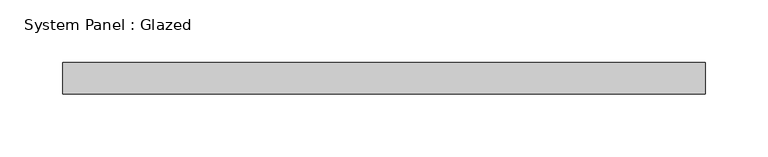
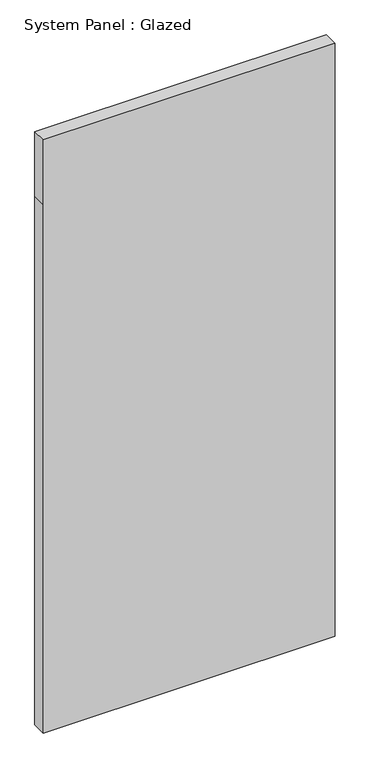
"""IFC4 building model written with IfcOpenShell, lengths in millimetres: plate geometry, System Panel : Glazed."""

from ifc_helpers import new_model, si_unit, frame, origin, place, context, project, spatial, polyline, outline, extrude, source, transform, mapped, element, save


def system_panel_glazed_a0a4d195(model_context):
    return source(origin(), model_context, "Body", "SweptSolid", [
        extrude(outline(polyline([(0.0, -257.175), (0.0, 257.175), (983.8490947, 257.175), (1104.4990947, 257.175), (1104.4990947, -257.175), (983.8490947, -257.175), (0.0, -257.175)])), frame((0.0, 19.05, 0.0), z_axis=(0.0, 1.0, 0.0), x_axis=(0.0, 0.0, 1.0)), (0.0, 0.0, 1.0), 25.4),
    ])


if __name__ == "__main__":
    model = new_model("IFC4")
    model_context = context("Model", 3, world=origin())
    ifc_project = project(units=[si_unit("LENGTHUNIT", "METRE", prefix="MILLI")], contexts=[model_context])
    site = spatial("IfcSite", under=ifc_project)
    building = spatial("IfcBuilding", under=site)
    placement = place(None, origin())
    system_panel_glazed_shape = system_panel_glazed_a0a4d195(model_context)
    element("IfcPlate", 1, ObjectType="System Panel : Glazed", at=placement, inside=building, context=model_context, shape_type="MappedRepresentation", body=[
        mapped(system_panel_glazed_shape, transform((0.0, 0.0, 0.0), x_axis=(1.0, 0.0, 0.0), y_axis=(0.0, 1.0, 0.0), z_axis=(0.0, 0.0, 1.0))),
    ])
    save(model, "model.ifc")

# Revit data of these elements
# Type "System Panel : Glazed"
#   Construction Type Id = "GSP4R"
#   Analytic Construction = "1/8 in Pilkington single glazing"
#   Visual Light Transmittance = 0.9
#   Solar Heat Gain Coefficient = 0.86
#   Heat Transfer Coefficient (U) = 1.18115 BTU/(h·ft²·°F)
#   Define Thermal Properties by = 1
# Element 1 (IfcPlate, "System Panel : Glazed")
#   Materials on its faces: "Glass"
# Materials
#   "Glass": class "Glass", colour RGB 0 128 192, transparency 0.75, Description = "Soda Lime Glass", Cost = 0
